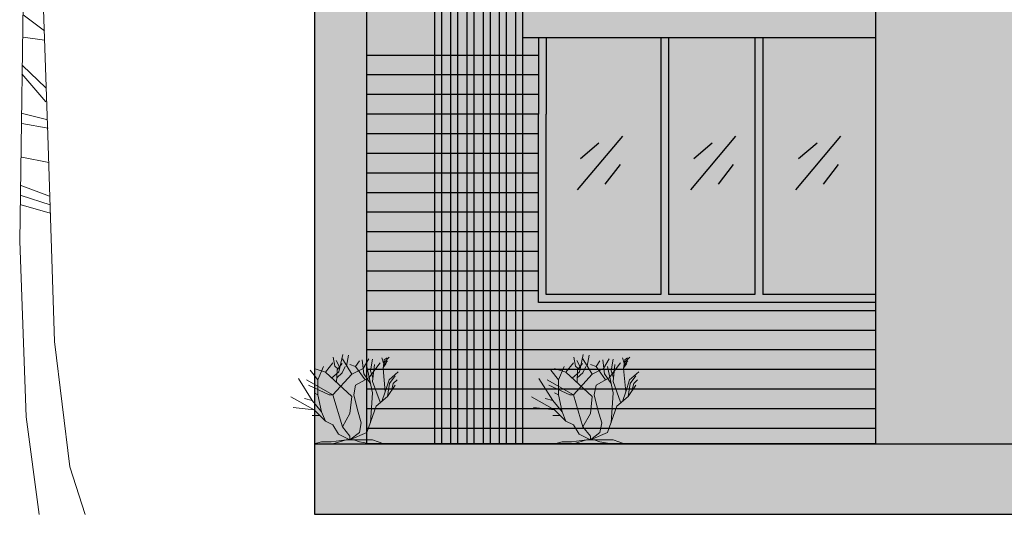
# Model space of a CAD drawing. Units: inches. Extents: x 13 to 1693, y -7 to 1519.
# Tile 5 of 10: x 41 to 292, y 1195 to 1321. Entities that reach past the tile are written whole.
import ezdxf

# ---------------------------------------------------------------- set-up
doc = ezdxf.new("R2010")
doc.units = ezdxf.units.IN
doc.header["$MEASUREMENT"] = 0
for name, color, linetype, lineweight in [('A-ELEV', 7, 'Continuous', 25), ('A-ELEV-PATT', 8, 'Continuous', 13), ('TREE', 102, 'Continuous', 18)]:
    doc.layers.add(name, color=color, linetype=linetype, lineweight=lineweight)

# ---------------------------------------------------------------- blocks, each defined once
blk = doc.blocks.new('*U29')
for p, q in [((-4.081, 127.298), (1.31, 123.246)), ((-4.081, 121.578), (1.31, 120.863)), ((-4.267, 114.428), (1.682, 108.708)), ((-4.453, 112.283), (1.682, 105.133)), ((-4.639, 102.273), (1.868, 100.604)), ((-4.453, 99.651), (2.24, 98.459)), ((-4.453, 91.071), (2.426, 89.641)), ((-4.825, 83.921), (2.612, 81.061)), ((-4.639, 81.299), (2.797, 78.916)), ((-4.639, 78.916), (2.797, 76.771))]:
    blk.add_line(p, q)
for points in [[(-2.363, 170.553), (-3.88, 148.505), (-4.988, 69.634), (-3.325, 24.869), (0, 0)], [(-0.116, 162.848), (0.554, 143.532), (2.217, 96.635), (3.88, 44.054), (7.76, 12.079), (11.64, 0)]]:
    blk.add_lwpolyline(points)
blk = doc.blocks.new('*U30')
for p, q in [((-11.433, 18.289), (-10.457, 22.749)), ((-9.48, 19.775), (-8.992, 22.592)), ((-14.88, 18.24), (-12.96, 20.64)), ((-12.471, 19.775), (-12.898, 22.044)), ((-11.28, 19.619), (-12.104, 21.184)), ((-11.921, 18.836), (-10.64, 20.401)), ((-8.16, 17.76), (-10.56, 21.6)), ((-7.2, 19.68), (-8.64, 20.16)), ((-7.2, 19.68), (-6.24, 21.12)), ((-5.086, 17.741), (-5.513, 21.34)), ((-5.28, 19.2), (-3.84, 21.6)), ((-3.84, 16.8), (-0.96, 20.64)), ((-3.377, 18.602), (-2.888, 21.575)), ((-2.88, 15.84), (-2.4, 20.16)), ((-0.508, 21.888), (-0.081, 20.558)), ((-0.203, 19.149), (0.102, 21.34)), ((-0.142, 19.384), (0.59, 20.401)), ((-0.02, 20.01), (0.896, 21.105)), ((0.041, 20.714), (1.384, 22.044)), ((0.102, 21.34), (0.835, 21.888)), ((-16.8, 16.32), (-18.72, 18.72)), ((-14.88, 18.24), (-17.76, 19.2)), ((-16.8, 16.32), (-15.36, 19.68)), ((-8.16, 12), (-14.88, 18.24)), ((-13.325, 16.724), (-11.433, 18.289)), ((-12.96, 12.48), (-8.16, 17.76)), ((-11.677, 19.071), (-12.471, 19.775)), ((-12.043, 15.628), (-11.921, 18.836)), ((-11.982, 16.802), (-10.579, 18.054)), ((-10.579, 18.054), (-9.846, 19.697)), ((-8.16, 17.76), (-5.28, 19.2)), ((-4.8, 16.32), (-7.2, 19.68)), ((-3.377, 15.315), (-5.086, 17.819)), ((-2.88, 12.96), (-4.32, 19.68)), ((-2.766, 16.802), (-3.377, 18.602)), ((0.346, 13.203), (-0.203, 19.149)), ((1.323, 16.254), (3.642, 18.289)), ((-18.24, 11.04), (-21.755, 16.655)), ((-12.96, 12.48), (-19.68, 16.32)), ((-16.8, 12.48), (-16.8, 16.32)), ((-7.2, 14.88), (-3.84, 16.8)), ((-0.96, 10.56), (-2.88, 15.84)), ((0.346, 13.203), (1.323, 16.254)), ((0.96, 12), (1.44, 15.36)), ((1.44, 15.36), (2.88, 17.28)), ((1.92, 13.44), (2.4, 15.36)), ((2.4, 15.36), (3.36, 16.32)), ((-13.92, 12.48), (-19.2, 14.88)), ((-16.8, 12.48), (-17.76, 12.96)), ((-7.68, 12.48), (-7.2, 14.88)), ((-3.36, 5.28), (-2.88, 12.96)), ((-0.48, 10.8), (0.346, 13.203)), ((0.96, 12), (2.88, 14.88)), ((-17.76, 8.64), (-23.663, 11.961)), ((-18.24, 11.04), (-20.16, 11.52)), ((-15.84, 8.16), (-18.24, 11.04)), ((-15.84, 8.16), (-16.8, 12.48)), ((-12.96, 12.48), (-13.92, 12.48)), ((-10.56, 4.32), (-12.96, 12.48)), ((-8.64, 7.68), (-8.16, 12)), ((-6.72, 8.64), (-7.68, 12.48)), ((-1.92, 9.6), (0.96, 12)), ((-17.76, 8.64), (-23.128, 9.222)), ((-14.88, 5.76), (-17.76, 8.64)), ((-14.88, 5.76), (-15.84, 8.16)), ((-10.56, 4.32), (-8.64, 7.68)), ((-5.76, 5.28), (-6.72, 8.64)), ((-4.32, 2.88), (-1.92, 9.6)), ((-16.32, 7.2), (-18.24, 7.2)), ((-12.96, 4.8), (-14.88, 5.76)), ((-6.24, 2.88), (-5.76, 5.28)), ((-11.52, 2.4), (-12.96, 4.8)), ((-8.64, 1.92), (-10.56, 4.32)), ((-8.64, 0.96), (-4.32, 2.88)), ((-8.64, 0.96), (-6.24, 2.88)), ((-15.84, 0.48), (-17.76, 0)), ((-13.44, 0.48), (-15.84, 0.48)), ((-9.6, 0.96), (-13.44, 0.48)), ((-9.6, 0.96), (-12.96, 0)), ((-8.64, 0.96), (-11.52, 2.4)), ((-9.6, 0.96), (-7.68, 0.96)), ((-8.64, 0.96), (-8.64, 1.92)), ((-8.64, 0.96), (-2.88, 0.96)), ((-7.68, 0.96), (-6.24, 0.48)), ((-6.24, 0.48), (-3.36, 0)), ((-2.88, 0.96), (0, 0))]:
    blk.add_line(p, q)

msp = doc.modelspace()

# ---------------------------------------------------------------- hatches: boundary and pattern name
at = {"layer": 'A-ELEV-PATT', "transparency": 33554664}
h = msp.add_hatch(color=256, dxfattribs=at)
h.dxf.hatch_style = 1
h.paths.add_polyline_path([(161.14, 1507.23), (159.26, 1507.23), (159.26, 1457.61), (161.14, 1457.61)])
h.paths.add_polyline_path([(161.14, 1510.4), (159.26, 1512.79), (159.26, 1507.23), (161.14, 1507.23)])
h.paths.add_polyline_path([(165.27, 1510.4), (163.39, 1512.79), (163.39, 1507.23), (165.27, 1507.23)])
h.paths.add_polyline_path([(169.4, 1510.4), (167.53, 1512.79), (167.53, 1507.23), (169.4, 1507.23)])
h.paths.add_polyline_path([(157.01, 1510.4), (155.13, 1512.79), (155.13, 1507.23), (157.01, 1507.23)])
h.paths.add_polyline_path([(152.87, 1510.4), (151, 1512.79), (151, 1507.23), (152.87, 1507.23)])
h.paths.add_polyline_path([(148.74, 1510.4), (146.87, 1512.79), (146.87, 1507.23), (148.74, 1507.23)])
h.paths.add_polyline_path([(148.74, 1507.23), (146.87, 1507.23), (146.87, 1457.61), (148.74, 1457.61)])
h.paths.add_polyline_path([(152.87, 1507.23), (151, 1507.23), (151, 1457.61), (152.87, 1457.61)])
h.paths.add_polyline_path([(157.01, 1507.23), (155.13, 1507.23), (155.13, 1457.61), (157.01, 1457.61)])
h.paths.add_polyline_path([(165.27, 1507.23), (163.39, 1507.23), (163.39, 1457.61), (165.27, 1457.61)])
h.paths.add_polyline_path([(169.4, 1507.23), (167.53, 1507.23), (167.53, 1457.61), (169.4, 1457.61)])
h.paths.add_polyline_path([(157.01, 1457.61), (155.13, 1457.61), (155.13, 1213.23), (157.01, 1213.23)])
h.paths.add_polyline_path([(161.14, 1457.61), (159.26, 1457.61), (159.26, 1213.23), (161.14, 1213.23)])
h.paths.add_polyline_path([(165.27, 1457.61), (163.39, 1457.61), (163.39, 1213.23), (165.27, 1213.23)])
h.paths.add_polyline_path([(169.4, 1457.61), (167.53, 1457.61), (167.53, 1213.23), (169.4, 1213.23)])
h.paths.add_polyline_path([(152.87, 1457.61), (151, 1457.61), (151, 1213.23), (152.87, 1213.23)])
h.paths.add_polyline_path([(148.74, 1457.61), (146.87, 1457.61), (146.87, 1213.23), (148.74, 1213.23)])
at = {"layer": 'A-ELEV-PATT'}
h = msp.add_hatch(color=256, dxfattribs=at)
h.dxf.hatch_style = 1
h.paths.add_polyline_path([(534.67, 1493.81), (311.73, 1493.81), (311.73, 1507.23), (169.4, 1507.23), (169.4, 1457.61), (259.19, 1457.61), (259.19, 1213.23), (294.63, 1213.23), (294.63, 1485.7), (299.21, 1485.7), (534.67, 1485.7)])
h.paths.add_polyline_path([(534.67, 1481.12), (299.21, 1481.12), (299.21, 1213.23), (314.45, 1213.23), (314.45, 1459.23), (520.13, 1459.23)], flags=17)
h.paths.add_polyline_path([(146.87, 1507.23), (116.45, 1507.23), (116.45, 1339.23), (116.45, 1213.23), (129.66, 1213.23), (129.66, 1457.61), (146.87, 1457.61)])
h.paths.add_polyline_path([(151, 1507.23), (148.74, 1507.23), (148.74, 1457.61), (151, 1457.61)])
h.paths.add_polyline_path([(155.13, 1507.23), (152.87, 1507.23), (152.87, 1457.61), (155.13, 1457.61)])
h.paths.add_polyline_path([(159.26, 1507.23), (157.01, 1507.23), (157.01, 1457.61), (159.26, 1457.61)])
h.paths.add_polyline_path([(163.39, 1507.23), (161.14, 1507.23), (161.14, 1457.61), (163.39, 1457.61)])
h.paths.add_polyline_path([(167.53, 1507.23), (165.27, 1507.23), (165.27, 1457.61), (167.53, 1457.61)])
h = msp.add_hatch(color=256, dxfattribs=at)
h.dxf.hatch_style = 1
h.paths.add_polyline_path([(259.19, 1457.61), (169.4, 1457.61), (169.4, 1453.8), (259.19, 1453.8)])
h.paths.add_polyline_path([(259.19, 1448.8), (169.4, 1448.8), (169.4, 1443.8), (259.19, 1443.8)])
h.paths.add_polyline_path([(259.19, 1438.8), (169.4, 1438.8), (169.4, 1433.8), (259.19, 1433.8)])
h.paths.add_polyline_path([(259.19, 1428.8), (169.4, 1428.8), (169.4, 1423.8), (259.19, 1423.8)])
h.paths.add_polyline_path([(146.87, 1457.61), (129.66, 1457.61), (129.66, 1453.8), (146.87, 1453.8)])
h.paths.add_polyline_path([(146.87, 1448.8), (129.66, 1448.8), (129.66, 1443.8), (146.87, 1443.8)])
h.paths.add_polyline_path([(146.87, 1438.8), (129.66, 1438.8), (129.66, 1433.8), (146.87, 1433.8)])
h.paths.add_polyline_path([(146.87, 1428.8), (129.66, 1428.8), (129.66, 1423.8), (146.87, 1423.8)])
h.paths.add_polyline_path([(151, 1457.61), (148.74, 1457.61), (148.74, 1453.8), (151, 1453.8)])
h.paths.add_polyline_path([(155.13, 1457.61), (152.87, 1457.61), (152.87, 1453.8), (155.13, 1453.8)])
h.paths.add_polyline_path([(159.26, 1457.61), (157.01, 1457.61), (157.01, 1453.8), (159.26, 1453.8)])
h.paths.add_polyline_path([(163.39, 1457.61), (161.14, 1457.61), (161.14, 1453.8), (163.39, 1453.8)])
h.paths.add_polyline_path([(167.53, 1457.61), (165.27, 1457.61), (165.27, 1453.8), (167.53, 1453.8)])
h.paths.add_polyline_path([(167.53, 1448.8), (165.27, 1448.8), (165.27, 1443.8), (167.53, 1443.8)])
h.paths.add_polyline_path([(163.39, 1448.8), (161.14, 1448.8), (161.14, 1443.8), (163.39, 1443.8)])
h.paths.add_polyline_path([(159.26, 1448.8), (157.01, 1448.8), (157.01, 1443.8), (159.26, 1443.8)])
h.paths.add_polyline_path([(155.13, 1448.8), (152.87, 1448.8), (152.87, 1443.8), (155.13, 1443.8)])
h.paths.add_polyline_path([(151, 1448.8), (148.74, 1448.8), (148.74, 1443.8), (151, 1443.8)])
h.paths.add_polyline_path([(151, 1438.8), (148.74, 1438.8), (148.74, 1433.8), (151, 1433.8)])
h.paths.add_polyline_path([(155.13, 1438.8), (152.87, 1438.8), (152.87, 1433.8), (155.13, 1433.8)])
h.paths.add_polyline_path([(159.26, 1438.8), (157.01, 1438.8), (157.01, 1433.8), (159.26, 1433.8)])
h.paths.add_polyline_path([(163.39, 1438.8), (161.14, 1438.8), (161.14, 1433.8), (163.39, 1433.8)])
h.paths.add_polyline_path([(167.53, 1438.8), (165.27, 1438.8), (165.27, 1433.8), (167.53, 1433.8)])
h.paths.add_polyline_path([(167.53, 1428.8), (165.27, 1428.8), (165.27, 1423.8), (167.53, 1423.8)])
h.paths.add_polyline_path([(163.39, 1428.8), (161.14, 1428.8), (161.14, 1423.8), (163.39, 1423.8)])
h.paths.add_polyline_path([(159.26, 1428.8), (157.01, 1428.8), (157.01, 1423.8), (159.26, 1423.8)])
h.paths.add_polyline_path([(155.13, 1428.8), (152.87, 1428.8), (152.87, 1423.8), (155.13, 1423.8)])
h.paths.add_polyline_path([(151, 1428.8), (148.74, 1428.8), (148.74, 1423.8), (151, 1423.8)])
h.paths.add_polyline_path([(146.87, 1418.8), (129.66, 1418.8), (129.66, 1413.8), (146.87, 1413.8)])
h.paths.add_polyline_path([(146.87, 1408.8), (129.66, 1408.8), (129.66, 1403.8), (146.87, 1403.8)])
h.paths.add_polyline_path([(146.87, 1398.8), (129.66, 1398.8), (129.66, 1393.8), (146.87, 1393.8)])
h.paths.add_polyline_path([(146.87, 1388.8), (129.66, 1388.8), (129.66, 1383.8), (146.87, 1383.8)])
h.paths.add_polyline_path([(146.87, 1378.8), (129.66, 1378.8), (129.66, 1373.8), (146.87, 1373.8)])
h.paths.add_polyline_path([(146.87, 1368.8), (129.66, 1368.8), (129.66, 1363.8), (146.87, 1363.8)])
h.paths.add_polyline_path([(146.87, 1358.8), (129.66, 1358.8), (129.66, 1353.8), (146.87, 1353.8)])
h.paths.add_polyline_path([(146.87, 1348.8), (129.66, 1348.8), (129.66, 1343.8), (146.87, 1343.8)])
h.paths.add_polyline_path([(146.87, 1338.8), (129.66, 1338.8), (129.66, 1333.8), (146.87, 1333.8)])
h.paths.add_polyline_path([(146.87, 1328.8), (129.66, 1328.8), (129.66, 1323.8), (146.87, 1323.8)])
h.paths.add_polyline_path([(146.87, 1318.8), (129.66, 1318.8), (129.66, 1312.21), (146.87, 1312.21)])
h.paths.add_polyline_path([(146.87, 1307.21), (129.66, 1307.21), (129.66, 1302.21), (146.87, 1302.21)])
h.paths.add_polyline_path([(146.87, 1297.21), (129.66, 1297.21), (129.66, 1292.21), (146.87, 1292.21)])
h.paths.add_polyline_path([(146.87, 1287.21), (129.66, 1287.21), (129.66, 1282.21), (146.87, 1282.21)])
h.paths.add_polyline_path([(146.87, 1277.21), (129.66, 1277.21), (129.66, 1272.21), (146.87, 1272.21)])
h.paths.add_polyline_path([(146.87, 1267.21), (129.66, 1267.21), (129.66, 1262.21), (146.87, 1262.21)])
h.paths.add_polyline_path([(146.87, 1257.21), (129.66, 1257.21), (129.66, 1252.21), (146.87, 1252.21)])
h.paths.add_polyline_path([(146.87, 1247.21), (129.66, 1247.21), (129.66, 1242.21), (146.87, 1242.21)])
h = msp.add_hatch(color=256, dxfattribs=at)
h.dxf.hatch_style = 1
h.paths.add_polyline_path([(259.19, 1453.8), (169.4, 1453.8), (169.4, 1448.8), (259.19, 1448.8)])
h.paths.add_polyline_path([(259.19, 1443.8), (169.4, 1443.8), (169.4, 1438.8), (259.19, 1438.8)])
h.paths.add_polyline_path([(259.19, 1433.8), (169.4, 1433.8), (169.4, 1428.8), (259.19, 1428.8)])
h.paths.add_polyline_path([(146.87, 1453.8), (129.66, 1453.8), (129.66, 1448.8), (146.87, 1448.8)])
h.paths.add_polyline_path([(146.87, 1443.8), (129.66, 1443.8), (129.66, 1438.8), (146.87, 1438.8)])
h.paths.add_polyline_path([(146.87, 1433.8), (129.66, 1433.8), (129.66, 1428.8), (146.87, 1428.8)])
h.paths.add_polyline_path([(146.87, 1423.8), (129.66, 1423.8), (129.66, 1418.8), (146.87, 1418.8)])
h.paths.add_polyline_path([(146.87, 1413.8), (129.66, 1413.8), (129.66, 1408.8), (146.87, 1408.8)])
h.paths.add_polyline_path([(146.87, 1403.8), (129.66, 1403.8), (129.66, 1398.8), (146.87, 1398.8)])
h.paths.add_polyline_path([(146.87, 1393.8), (129.66, 1393.8), (129.66, 1388.8), (146.87, 1388.8)])
h.paths.add_polyline_path([(146.87, 1383.8), (129.66, 1383.8), (129.66, 1378.8), (146.87, 1378.8)])
h.paths.add_polyline_path([(146.87, 1373.8), (129.66, 1373.8), (129.66, 1368.8), (146.87, 1368.8)])
h.paths.add_polyline_path([(146.87, 1363.8), (129.66, 1363.8), (129.66, 1358.8), (146.87, 1358.8)])
h.paths.add_polyline_path([(146.87, 1353.8), (129.66, 1353.8), (129.66, 1348.8), (146.87, 1348.8)])
h.paths.add_polyline_path([(146.87, 1343.8), (129.66, 1343.8), (129.66, 1338.8), (146.87, 1338.8)])
h.paths.add_polyline_path([(146.87, 1333.8), (129.66, 1333.8), (129.66, 1328.8), (146.87, 1328.8)])
h.paths.add_polyline_path([(146.87, 1323.8), (129.66, 1323.8), (129.66, 1318.8), (146.87, 1318.8)])
h.paths.add_polyline_path([(146.87, 1312.21), (129.66, 1312.21), (129.66, 1307.21), (146.87, 1307.21)])
h.paths.add_polyline_path([(146.87, 1302.21), (129.66, 1302.21), (129.66, 1297.21), (146.87, 1297.21)])
h.paths.add_polyline_path([(146.87, 1292.21), (129.66, 1292.21), (129.66, 1287.21), (146.87, 1287.21)])
h.paths.add_polyline_path([(146.87, 1282.21), (129.66, 1282.21), (129.66, 1277.21), (146.87, 1277.21)])
h.paths.add_polyline_path([(146.87, 1272.21), (129.66, 1272.21), (129.66, 1267.21), (146.87, 1267.21)])
h.paths.add_polyline_path([(146.87, 1262.21), (129.66, 1262.21), (129.66, 1257.21), (146.87, 1257.21)])
h.paths.add_polyline_path([(146.87, 1252.21), (129.66, 1252.21), (129.66, 1247.21), (146.87, 1247.21)])
h.paths.add_polyline_path([(146.87, 1242.21), (129.66, 1242.21), (129.66, 1237.21), (146.87, 1237.21)])
h.paths.add_polyline_path([(146.87, 1232.21), (129.66, 1232.21), (129.66, 1227.21), (146.87, 1227.21)])
h.paths.add_polyline_path([(146.87, 1222.21), (129.66, 1222.21), (129.66, 1217.21), (146.87, 1217.21)])
h.paths.add_polyline_path([(259.19, 1242.21), (169.4, 1242.21), (169.4, 1237.21), (259.19, 1237.21)])
h.paths.add_polyline_path([(259.19, 1232.21), (169.4, 1232.21), (169.4, 1227.21), (259.19, 1227.21)])
h.paths.add_polyline_path([(259.19, 1222.21), (169.4, 1222.21), (169.4, 1217.21), (259.19, 1217.21)])
h = msp.add_hatch(color=256, dxfattribs=at)
h.dxf.hatch_style = 1
h.paths.add_polyline_path([(173.34, 1282.21), (169.4, 1282.21), (169.4, 1277.21), (173.34, 1277.21)])
h.paths.add_polyline_path([(173.34, 1292.21), (169.4, 1292.21), (169.4, 1287.21), (173.34, 1287.21)])
h.paths.add_polyline_path([(173.34, 1272.21), (169.4, 1272.21), (169.4, 1267.21), (173.34, 1267.21)])
h.paths.add_polyline_path([(173.34, 1262.21), (169.4, 1262.21), (169.4, 1257.21), (173.34, 1257.21)])
h.paths.add_polyline_path([(173.34, 1312.21), (169.4, 1312.21), (169.4, 1307.21), (173.34, 1307.21)])
h.paths.add_polyline_path([(173.34, 1302.21), (169.4, 1302.21), (169.4, 1297.21), (173.34, 1297.21)])
h.paths.add_polyline_path([(167.53, 1323.8), (165.27, 1323.8), (165.27, 1318.8), (167.53, 1318.8)])
h.paths.add_polyline_path([(167.53, 1333.8), (165.27, 1333.8), (165.27, 1328.8), (167.53, 1328.8)])
h.paths.add_polyline_path([(163.39, 1333.8), (161.14, 1333.8), (161.14, 1328.8), (163.39, 1328.8)])
h.paths.add_polyline_path([(159.26, 1333.8), (157.01, 1333.8), (157.01, 1328.8), (159.26, 1328.8)])
h.paths.add_polyline_path([(155.13, 1333.8), (152.87, 1333.8), (152.87, 1328.8), (155.13, 1328.8)])
h.paths.add_polyline_path([(151, 1333.8), (148.74, 1333.8), (148.74, 1328.8), (151, 1328.8)])
h.paths.add_polyline_path([(151, 1323.8), (148.74, 1323.8), (148.74, 1318.8), (151, 1318.8)])
h.paths.add_polyline_path([(155.13, 1323.8), (152.87, 1323.8), (152.87, 1318.8), (155.13, 1318.8)])
h.paths.add_polyline_path([(159.26, 1323.8), (157.01, 1323.8), (157.01, 1318.8), (159.26, 1318.8)])
h.paths.add_polyline_path([(163.39, 1323.8), (161.14, 1323.8), (161.14, 1318.8), (163.39, 1318.8)])
h.paths.add_polyline_path([(163.39, 1312.21), (161.14, 1312.21), (161.14, 1307.21), (163.39, 1307.21)])
h.paths.add_polyline_path([(167.53, 1312.21), (165.27, 1312.21), (165.27, 1307.21), (167.53, 1307.21)])
h.paths.add_polyline_path([(167.53, 1302.21), (165.27, 1302.21), (165.27, 1297.21), (167.53, 1297.21)])
h.paths.add_polyline_path([(167.53, 1292.21), (165.27, 1292.21), (165.27, 1287.21), (167.53, 1287.21)])
h.paths.add_polyline_path([(163.39, 1292.21), (161.14, 1292.21), (161.14, 1287.21), (163.39, 1287.21)])
h.paths.add_polyline_path([(163.39, 1302.21), (161.14, 1302.21), (161.14, 1297.21), (163.39, 1297.21)])
h.paths.add_polyline_path([(159.26, 1302.21), (157.01, 1302.21), (157.01, 1297.21), (159.26, 1297.21)])
h.paths.add_polyline_path([(159.26, 1312.21), (157.01, 1312.21), (157.01, 1307.21), (159.26, 1307.21)])
h.paths.add_polyline_path([(155.13, 1312.21), (152.87, 1312.21), (152.87, 1307.21), (155.13, 1307.21)])
h.paths.add_polyline_path([(151, 1312.21), (148.74, 1312.21), (148.74, 1307.21), (151, 1307.21)])
h.paths.add_polyline_path([(151, 1302.21), (148.74, 1302.21), (148.74, 1297.21), (151, 1297.21)])
h.paths.add_polyline_path([(155.13, 1302.21), (152.87, 1302.21), (152.87, 1297.21), (155.13, 1297.21)])
h.paths.add_polyline_path([(155.13, 1292.21), (152.87, 1292.21), (152.87, 1287.21), (155.13, 1287.21)])
h.paths.add_polyline_path([(151, 1292.21), (148.74, 1292.21), (148.74, 1287.21), (151, 1287.21)])
h.paths.add_polyline_path([(159.26, 1292.21), (157.01, 1292.21), (157.01, 1287.21), (159.26, 1287.21)])
h.paths.add_polyline_path([(159.26, 1282.21), (157.01, 1282.21), (157.01, 1277.21), (159.26, 1277.21)])
h.paths.add_polyline_path([(163.39, 1282.21), (161.14, 1282.21), (161.14, 1277.21), (163.39, 1277.21)])
h.paths.add_polyline_path([(167.53, 1282.21), (165.27, 1282.21), (165.27, 1277.21), (167.53, 1277.21)])
h.paths.add_polyline_path([(155.13, 1282.21), (152.87, 1282.21), (152.87, 1277.21), (155.13, 1277.21)])
h.paths.add_polyline_path([(151, 1282.21), (148.74, 1282.21), (148.74, 1277.21), (151, 1277.21)])
h.paths.add_polyline_path([(151, 1272.21), (148.74, 1272.21), (148.74, 1267.21), (151, 1267.21)])
h.paths.add_polyline_path([(155.13, 1272.21), (152.87, 1272.21), (152.87, 1267.21), (155.13, 1267.21)])
h.paths.add_polyline_path([(159.26, 1272.21), (157.01, 1272.21), (157.01, 1267.21), (159.26, 1267.21)])
h.paths.add_polyline_path([(163.39, 1272.21), (161.14, 1272.21), (161.14, 1267.21), (163.39, 1267.21)])
h.paths.add_polyline_path([(167.53, 1272.21), (165.27, 1272.21), (165.27, 1267.21), (167.53, 1267.21)])
h.paths.add_polyline_path([(167.53, 1262.21), (165.27, 1262.21), (165.27, 1257.21), (167.53, 1257.21)])
h.paths.add_polyline_path([(163.39, 1262.21), (161.14, 1262.21), (161.14, 1257.21), (163.39, 1257.21)])
h.paths.add_polyline_path([(163.39, 1252.21), (161.14, 1252.21), (161.14, 1247.21), (163.39, 1247.21)])
h.paths.add_polyline_path([(159.26, 1252.21), (157.01, 1252.21), (157.01, 1247.21), (159.26, 1247.21)])
h.paths.add_polyline_path([(159.26, 1262.21), (157.01, 1262.21), (157.01, 1257.21), (159.26, 1257.21)])
h.paths.add_polyline_path([(155.13, 1262.21), (152.87, 1262.21), (152.87, 1257.21), (155.13, 1257.21)])
h.paths.add_polyline_path([(151, 1262.21), (148.74, 1262.21), (148.74, 1257.21), (151, 1257.21)])
h.paths.add_polyline_path([(151, 1252.21), (148.74, 1252.21), (148.74, 1247.21), (151, 1247.21)])
h.paths.add_polyline_path([(155.13, 1252.21), (152.87, 1252.21), (152.87, 1247.21), (155.13, 1247.21)])
h.paths.add_polyline_path([(151, 1242.21), (148.74, 1242.21), (148.74, 1237.21), (151, 1237.21)])
h.paths.add_polyline_path([(155.13, 1242.21), (152.87, 1242.21), (152.87, 1237.21), (155.13, 1237.21)])
h.paths.add_polyline_path([(159.26, 1242.21), (157.01, 1242.21), (157.01, 1237.21), (159.26, 1237.21)])
h.paths.add_polyline_path([(163.39, 1242.21), (161.14, 1242.21), (161.14, 1237.21), (163.39, 1237.21)])
h.paths.add_polyline_path([(173.34, 1363.8), (169.4, 1363.8), (169.4, 1358.8), (173.34, 1358.8)])
h.paths.add_polyline_path([(173.34, 1373.8), (169.4, 1373.8), (169.4, 1368.8), (173.34, 1368.8)])
h.paths.add_polyline_path([(173.34, 1381.23), (173.34, 1383.8), (169.4, 1383.8), (169.4, 1378.8), (173.34, 1378.8)])
h.paths.add_polyline_path([(173.34, 1393.8), (169.4, 1393.8), (169.4, 1388.8), (173.34, 1388.8)])
h.paths.add_polyline_path([(173.34, 1403.8), (169.4, 1403.8), (169.4, 1398.8), (173.34, 1398.8)])
h.paths.add_polyline_path([(173.34, 1413.8), (169.4, 1413.8), (169.4, 1408.8), (173.34, 1408.8)])
h.paths.add_polyline_path([(167.53, 1383.8), (165.27, 1383.8), (165.27, 1378.8), (167.53, 1378.8)])
h.paths.add_polyline_path([(167.53, 1373.8), (165.27, 1373.8), (165.27, 1368.8), (167.53, 1368.8)])
h.paths.add_polyline_path([(167.53, 1363.8), (165.27, 1363.8), (165.27, 1358.8), (167.53, 1358.8)])
h.paths.add_polyline_path([(167.53, 1353.8), (165.27, 1353.8), (165.27, 1348.8), (167.53, 1348.8)])
h.paths.add_polyline_path([(163.39, 1353.8), (161.14, 1353.8), (161.14, 1348.8), (163.39, 1348.8)])
h.paths.add_polyline_path([(163.39, 1363.8), (161.14, 1363.8), (161.14, 1358.8), (163.39, 1358.8)])
h.paths.add_polyline_path([(163.39, 1373.8), (161.14, 1373.8), (161.14, 1368.8), (163.39, 1368.8)])
h.paths.add_polyline_path([(163.39, 1383.8), (161.14, 1383.8), (161.14, 1378.8), (163.39, 1378.8)])
h.paths.add_polyline_path([(163.39, 1393.8), (161.14, 1393.8), (161.14, 1388.8), (163.39, 1388.8)])
h.paths.add_polyline_path([(163.39, 1403.8), (161.14, 1403.8), (161.14, 1398.8), (163.39, 1398.8)])
h.paths.add_polyline_path([(167.53, 1403.8), (165.27, 1403.8), (165.27, 1398.8), (167.53, 1398.8)])
h.paths.add_polyline_path([(167.53, 1393.8), (165.27, 1393.8), (165.27, 1388.8), (167.53, 1388.8)])
h.paths.add_polyline_path([(167.53, 1413.8), (165.27, 1413.8), (165.27, 1408.8), (167.53, 1408.8)])
h.paths.add_polyline_path([(163.39, 1413.8), (161.14, 1413.8), (161.14, 1408.8), (163.39, 1408.8)])
h.paths.add_polyline_path([(159.26, 1413.8), (157.01, 1413.8), (157.01, 1408.8), (159.26, 1408.8)])
h.paths.add_polyline_path([(155.13, 1413.8), (152.87, 1413.8), (152.87, 1408.8), (155.13, 1408.8)])
h.paths.add_polyline_path([(151, 1413.8), (148.74, 1413.8), (148.74, 1408.8), (151, 1408.8)])
h.paths.add_polyline_path([(151, 1403.8), (148.74, 1403.8), (148.74, 1398.8), (151, 1398.8)])
h.paths.add_polyline_path([(155.13, 1403.8), (152.87, 1403.8), (152.87, 1398.8), (155.13, 1398.8)])
h.paths.add_polyline_path([(159.26, 1403.8), (157.01, 1403.8), (157.01, 1398.8), (159.26, 1398.8)])
h.paths.add_polyline_path([(159.26, 1393.8), (157.01, 1393.8), (157.01, 1388.8), (159.26, 1388.8)])
h.paths.add_polyline_path([(155.13, 1393.8), (152.87, 1393.8), (152.87, 1388.8), (155.13, 1388.8)])
h.paths.add_polyline_path([(151, 1393.8), (148.74, 1393.8), (148.74, 1388.8), (151, 1388.8)])
h.paths.add_polyline_path([(151, 1383.8), (148.74, 1383.8), (148.74, 1378.8), (151, 1378.8)])
h.paths.add_polyline_path([(155.13, 1383.8), (152.87, 1383.8), (152.87, 1378.8), (155.13, 1378.8)])
h.paths.add_polyline_path([(159.26, 1383.8), (157.01, 1383.8), (157.01, 1378.8), (159.26, 1378.8)])
h.paths.add_polyline_path([(159.26, 1373.8), (157.01, 1373.8), (157.01, 1368.8), (159.26, 1368.8)])
h.paths.add_polyline_path([(155.13, 1373.8), (152.87, 1373.8), (152.87, 1368.8), (155.13, 1368.8)])
h.paths.add_polyline_path([(151, 1373.8), (148.74, 1373.8), (148.74, 1368.8), (151, 1368.8)])
h.paths.add_polyline_path([(151, 1363.8), (148.74, 1363.8), (148.74, 1358.8), (151, 1358.8)])
h.paths.add_polyline_path([(155.13, 1363.8), (152.87, 1363.8), (152.87, 1358.8), (155.13, 1358.8)])
h.paths.add_polyline_path([(159.26, 1363.8), (157.01, 1363.8), (157.01, 1358.8), (159.26, 1358.8)])
h.paths.add_polyline_path([(159.26, 1353.8), (157.01, 1353.8), (157.01, 1348.8), (159.26, 1348.8)])
h.paths.add_polyline_path([(155.13, 1353.8), (152.87, 1353.8), (152.87, 1348.8), (155.13, 1348.8)])
h.paths.add_polyline_path([(151, 1353.8), (148.74, 1353.8), (148.74, 1348.8), (151, 1348.8)])
h.paths.add_polyline_path([(151, 1343.8), (148.74, 1343.8), (148.74, 1338.8), (151, 1338.8)])
h.paths.add_polyline_path([(155.13, 1343.8), (152.87, 1343.8), (152.87, 1338.8), (155.13, 1338.8)])
h.paths.add_polyline_path([(159.26, 1343.8), (157.01, 1343.8), (157.01, 1338.8), (159.26, 1338.8)])
h.paths.add_polyline_path([(163.39, 1343.8), (161.14, 1343.8), (161.14, 1338.8), (163.39, 1338.8)])
h.paths.add_polyline_path([(167.53, 1343.8), (165.27, 1343.8), (165.27, 1338.8), (167.53, 1338.8)])
h.paths.add_polyline_path([(151, 1453.8), (148.74, 1453.8), (148.74, 1448.8), (151, 1448.8)])
h.paths.add_polyline_path([(155.13, 1453.8), (152.87, 1453.8), (152.87, 1448.8), (155.13, 1448.8)])
h.paths.add_polyline_path([(159.26, 1453.8), (157.01, 1453.8), (157.01, 1448.8), (159.26, 1448.8)])
h.paths.add_polyline_path([(163.39, 1453.8), (161.14, 1453.8), (161.14, 1448.8), (163.39, 1448.8)])
h.paths.add_polyline_path([(167.53, 1453.8), (165.27, 1453.8), (165.27, 1448.8), (167.53, 1448.8)])
h.paths.add_polyline_path([(167.53, 1443.8), (165.27, 1443.8), (165.27, 1438.8), (167.53, 1438.8)])
h.paths.add_polyline_path([(163.39, 1443.8), (161.14, 1443.8), (161.14, 1438.8), (163.39, 1438.8)])
h.paths.add_polyline_path([(159.26, 1443.8), (157.01, 1443.8), (157.01, 1438.8), (159.26, 1438.8)])
h.paths.add_polyline_path([(155.13, 1443.8), (152.87, 1443.8), (152.87, 1438.8), (155.13, 1438.8)])
h.paths.add_polyline_path([(151, 1443.8), (148.74, 1443.8), (148.74, 1438.8), (151, 1438.8)])
h.paths.add_polyline_path([(151, 1433.8), (148.74, 1433.8), (148.74, 1428.8), (151, 1428.8)])
h.paths.add_polyline_path([(155.13, 1433.8), (152.87, 1433.8), (152.87, 1428.8), (155.13, 1428.8)])
h.paths.add_polyline_path([(159.26, 1433.8), (157.01, 1433.8), (157.01, 1428.8), (159.26, 1428.8)])
h.paths.add_polyline_path([(163.39, 1433.8), (161.14, 1433.8), (161.14, 1428.8), (163.39, 1428.8)])
h.paths.add_polyline_path([(167.53, 1433.8), (165.27, 1433.8), (165.27, 1428.8), (167.53, 1428.8)])
h.paths.add_polyline_path([(173.34, 1423.23), (249.37, 1423.23), (259.19, 1423.23), (259.19, 1423.8), (169.4, 1423.8), (169.4, 1418.8), (173.34, 1418.8)])
h.paths.add_polyline_path([(167.53, 1423.8), (165.27, 1423.8), (165.27, 1418.8), (167.53, 1418.8)])
h.paths.add_polyline_path([(163.39, 1423.8), (161.14, 1423.8), (161.14, 1418.8), (163.39, 1418.8)])
h.paths.add_polyline_path([(159.26, 1423.8), (157.01, 1423.8), (157.01, 1418.8), (159.26, 1418.8)])
h.paths.add_polyline_path([(155.13, 1423.8), (152.87, 1423.8), (152.87, 1418.8), (155.13, 1418.8)])
h.paths.add_polyline_path([(151, 1423.8), (148.74, 1423.8), (148.74, 1418.8), (151, 1418.8)])
at = {"layer": 'A-ELEV-PATT', "transparency": 33554592}
h = msp.add_hatch(color=256, dxfattribs=at)
h.dxf.hatch_style = 1
h.paths.add_polyline_path([(202.48, 1421.23), (175.34, 1421.23), (175.34, 1381.23), (175.34, 1354.34), (202.48, 1354.34)])
h.paths.add_polyline_path([(226.48, 1421.23), (211.36, 1421.23), (204.48, 1421.23), (204.48, 1354.34), (226.48, 1354.34)])
h.paths.add_polyline_path([(259.19, 1421.23), (228.48, 1421.23), (228.48, 1354.34), (259.19, 1354.34)])
h.paths.add_polyline_path([(259.19, 1316.67), (230.48, 1316.67), (230.48, 1251.23), (259.19, 1251.23)])
h.paths.add_polyline_path([(228.48, 1316.67), (206.48, 1316.67), (206.48, 1251.23), (228.48, 1251.23)])
h.paths.add_polyline_path([(204.48, 1316.67), (175.34, 1316.67), (175.34, 1297.23), (175.34, 1251.23), (204.48, 1251.23)])
h.paths.add_polyline_path([(480.46, 1381.23), (476.14, 1387.14), (476.14, 1345.14), (480.46, 1339.23)])
h.paths.add_polyline_path([(683.45, 1381.23), (480.46, 1381.23), (480.46, 1339.23), (683.45, 1339.23)])
h.paths.add_polyline_path([(348.45, 1421.23), (325.77, 1421.23), (325.77, 1356.34), (348.45, 1356.34)])
h.paths.add_polyline_path([(474.14, 1421.23), (451.45, 1421.23), (451.45, 1356.34), (474.14, 1356.34)])
h.paths.add_polyline_path([(474.14, 1354.34), (451.45, 1354.34), (451.45, 1316.67), (474.14, 1316.67)])
h.paths.add_polyline_path([(348.45, 1354.34), (325.77, 1354.34), (325.77, 1316.67), (348.45, 1316.67)])
h.paths.add_polyline_path([(348.45, 1314.67), (325.77, 1314.67), (325.77, 1215.23), (348.45, 1215.23)])
h.paths.add_polyline_path([(474.14, 1314.67), (451.45, 1314.67), (451.45, 1215.23), (474.14, 1215.23)])
at = {"layer": 'A-ELEV-PATT'}
h = msp.add_hatch(color=256, dxfattribs=at)
h.dxf.hatch_style = 1
h.paths.add_polyline_path([(146.87, 1237.21), (129.66, 1237.21), (129.66, 1232.21), (146.87, 1232.21)])
h.paths.add_polyline_path([(146.87, 1227.21), (129.66, 1227.21), (129.66, 1222.21), (146.87, 1222.21)])
h.paths.add_polyline_path([(146.87, 1217.21), (129.66, 1217.21), (129.66, 1213.23), (146.87, 1213.23)])
h.paths.add_polyline_path([(259.19, 1217.21), (169.4, 1217.21), (169.4, 1213.23), (259.19, 1213.23)])
h.paths.add_polyline_path([(259.19, 1227.21), (169.4, 1227.21), (169.4, 1222.21), (259.19, 1222.21)])
h.paths.add_polyline_path([(259.19, 1237.21), (169.4, 1237.21), (169.4, 1232.21), (259.19, 1232.21)])
h.paths.add_polyline_path([(259.19, 1247.21), (169.4, 1247.21), (169.4, 1242.21), (259.19, 1242.21)])
h.paths.add_polyline_path([(173.34, 1257.21), (169.4, 1257.21), (169.4, 1252.21), (173.34, 1252.21)])
h.paths.add_polyline_path([(173.34, 1267.21), (169.4, 1267.21), (169.4, 1262.21), (173.34, 1262.21)])
h.paths.add_polyline_path([(173.34, 1277.21), (169.4, 1277.21), (169.4, 1272.21), (173.34, 1272.21)])
h.paths.add_polyline_path([(173.34, 1287.21), (169.4, 1287.21), (169.4, 1282.21), (173.34, 1282.21)])
h.paths.add_polyline_path([(173.34, 1297.21), (169.4, 1297.21), (169.4, 1292.21), (173.34, 1292.21)])
h.paths.add_polyline_path([(173.34, 1307.21), (169.4, 1307.21), (169.4, 1302.21), (173.34, 1302.21)])
h.paths.add_polyline_path([(173.34, 1316.67), (169.4, 1316.67), (169.4, 1312.21), (173.34, 1312.21)])
h.paths.add_polyline_path([(173.34, 1358.8), (169.4, 1358.8), (169.4, 1354.34), (173.34, 1354.34)])
h.paths.add_polyline_path([(173.34, 1368.8), (169.4, 1368.8), (169.4, 1363.8), (173.34, 1363.8)])
h.paths.add_polyline_path([(173.34, 1378.8), (169.4, 1378.8), (169.4, 1373.8), (173.34, 1373.8)])
h.paths.add_polyline_path([(173.34, 1388.8), (169.4, 1388.8), (169.4, 1383.8), (173.34, 1383.8)])
h = msp.add_hatch(color=256, dxfattribs=at)
h.dxf.hatch_style = 1
h.paths.add_polyline_path([(259.19, 1354.34), (169.4, 1354.34), (169.4, 1316.67), (259.19, 1316.67)])
h = msp.add_hatch(color=256, dxfattribs=at)
h.dxf.hatch_style = 1
h.paths.add_polyline_path([(151, 1318.8), (148.74, 1318.8), (148.74, 1312.21), (151, 1312.21)])
h.paths.add_polyline_path([(155.13, 1318.8), (152.87, 1318.8), (152.87, 1312.21), (155.13, 1312.21)])
h.paths.add_polyline_path([(159.26, 1318.8), (157.01, 1318.8), (157.01, 1312.21), (159.26, 1312.21)])
h.paths.add_polyline_path([(163.39, 1318.8), (161.14, 1318.8), (161.14, 1312.21), (163.39, 1312.21)])
h.paths.add_polyline_path([(167.53, 1318.8), (165.27, 1318.8), (165.27, 1312.21), (167.53, 1312.21)])
h = msp.add_hatch(color=256, dxfattribs=at)
h.dxf.hatch_style = 1
h.paths.add_polyline_path([(175.34, 1297.23), (175.34, 1316.67), (173.34, 1316.67), (173.34, 1297.23), (173.34, 1249.23), (259.19, 1249.23), (259.19, 1251.23), (230.48, 1251.23), (230.48, 1316.67), (228.48, 1316.67), (228.48, 1251.23), (206.48, 1251.23), (206.48, 1316.67), (204.48, 1316.67), (204.48, 1251.23), (175.34, 1251.23)])
h = msp.add_hatch(color=256, dxfattribs=at)
h.dxf.hatch_style = 1
h.paths.add_polyline_path([(167.53, 1307.21), (165.27, 1307.21), (165.27, 1302.21), (167.53, 1302.21)])
h.paths.add_polyline_path([(163.39, 1307.21), (161.14, 1307.21), (161.14, 1302.21), (163.39, 1302.21)])
h.paths.add_polyline_path([(159.26, 1307.21), (157.01, 1307.21), (157.01, 1302.21), (159.26, 1302.21)])
h.paths.add_polyline_path([(155.13, 1307.21), (152.87, 1307.21), (152.87, 1302.21), (155.13, 1302.21)])
h.paths.add_polyline_path([(151, 1307.21), (148.74, 1307.21), (148.74, 1302.21), (151, 1302.21)])
h = msp.add_hatch(color=256, dxfattribs=at)
h.dxf.hatch_style = 1
h.paths.add_polyline_path([(151, 1297.21), (148.74, 1297.21), (148.74, 1292.21), (151, 1292.21)])
h.paths.add_polyline_path([(155.13, 1297.21), (152.87, 1297.21), (152.87, 1292.21), (155.13, 1292.21)])
h.paths.add_polyline_path([(159.26, 1297.21), (157.01, 1297.21), (157.01, 1292.21), (159.26, 1292.21)])
h.paths.add_polyline_path([(163.39, 1297.21), (161.14, 1297.21), (161.14, 1292.21), (163.39, 1292.21)])
h.paths.add_polyline_path([(167.53, 1297.21), (165.27, 1297.21), (165.27, 1292.21), (167.53, 1292.21)])
h = msp.add_hatch(color=256, dxfattribs=at)
h.dxf.hatch_style = 1
h.paths.add_polyline_path([(167.53, 1287.21), (165.27, 1287.21), (165.27, 1282.21), (167.53, 1282.21)])
h.paths.add_polyline_path([(163.39, 1287.21), (161.14, 1287.21), (161.14, 1282.21), (163.39, 1282.21)])
h.paths.add_polyline_path([(159.26, 1287.21), (157.01, 1287.21), (157.01, 1282.21), (159.26, 1282.21)])
h.paths.add_polyline_path([(155.13, 1287.21), (152.87, 1287.21), (152.87, 1282.21), (155.13, 1282.21)])
h.paths.add_polyline_path([(151, 1287.21), (148.74, 1287.21), (148.74, 1282.21), (151, 1282.21)])
h.paths.add_polyline_path([(151, 1277.21), (148.74, 1277.21), (148.74, 1272.21), (151, 1272.21)])
h.paths.add_polyline_path([(155.13, 1277.21), (152.87, 1277.21), (152.87, 1272.21), (155.13, 1272.21)])
h.paths.add_polyline_path([(159.26, 1277.21), (157.01, 1277.21), (157.01, 1272.21), (159.26, 1272.21)])
h.paths.add_polyline_path([(163.39, 1277.21), (161.14, 1277.21), (161.14, 1272.21), (163.39, 1272.21)])
h.paths.add_polyline_path([(167.53, 1277.21), (165.27, 1277.21), (165.27, 1272.21), (167.53, 1272.21)])
h = msp.add_hatch(color=256, dxfattribs=at)
h.dxf.hatch_style = 1
h.paths.add_polyline_path([(163.39, 1247.21), (161.14, 1247.21), (161.14, 1242.21), (163.39, 1242.21)])
h.paths.add_polyline_path([(163.39, 1257.21), (161.14, 1257.21), (161.14, 1252.21), (163.39, 1252.21)])
h.paths.add_polyline_path([(163.39, 1267.21), (161.14, 1267.21), (161.14, 1262.21), (163.39, 1262.21)])
h.paths.add_polyline_path([(159.26, 1267.21), (157.01, 1267.21), (157.01, 1262.21), (159.26, 1262.21)])
h.paths.add_polyline_path([(155.13, 1267.21), (152.87, 1267.21), (152.87, 1262.21), (155.13, 1262.21)])
h.paths.add_polyline_path([(151, 1267.21), (148.74, 1267.21), (148.74, 1262.21), (151, 1262.21)])
h.paths.add_polyline_path([(151, 1257.21), (148.74, 1257.21), (148.74, 1252.21), (151, 1252.21)])
h.paths.add_polyline_path([(151, 1247.21), (148.74, 1247.21), (148.74, 1242.21), (151, 1242.21)])
h.paths.add_polyline_path([(155.13, 1247.21), (152.87, 1247.21), (152.87, 1242.21), (155.13, 1242.21)])
h.paths.add_polyline_path([(155.13, 1257.21), (152.87, 1257.21), (152.87, 1252.21), (155.13, 1252.21)])
h.paths.add_polyline_path([(159.26, 1257.21), (157.01, 1257.21), (157.01, 1252.21), (159.26, 1252.21)])
h.paths.add_polyline_path([(159.26, 1247.21), (157.01, 1247.21), (157.01, 1242.21), (159.26, 1242.21)])
h = msp.add_hatch(color=256, dxfattribs=at)
h.dxf.hatch_style = 1
h.paths.add_polyline_path([(167.53, 1267.21), (165.27, 1267.21), (165.27, 1262.21), (167.53, 1262.21)])
h.paths.add_polyline_path([(167.53, 1257.21), (165.27, 1257.21), (165.27, 1252.21), (167.53, 1252.21)])
h.paths.add_polyline_path([(167.53, 1247.21), (165.27, 1247.21), (165.27, 1242.21), (167.53, 1242.21)])
h = msp.add_hatch(color=256, dxfattribs=at)
h.dxf.hatch_style = 1
h.paths.add_polyline_path([(259.19, 1249.23), (173.34, 1249.23), (173.34, 1252.21), (169.4, 1252.21), (169.4, 1247.21), (259.19, 1247.21)])
h.paths.add_polyline_path([(167.53, 1252.21), (165.27, 1252.21), (165.27, 1247.21), (167.53, 1247.21)])
h.paths.add_polyline_path([(167.53, 1242.21), (165.27, 1242.21), (165.27, 1237.21), (167.53, 1237.21)])
h.paths.add_polyline_path([(167.53, 1232.21), (165.27, 1232.21), (165.27, 1227.21), (167.53, 1227.21)])
h.paths.add_polyline_path([(167.53, 1222.21), (165.27, 1222.21), (165.27, 1217.21), (167.53, 1217.21)])
h.paths.add_polyline_path([(163.39, 1222.21), (161.14, 1222.21), (161.14, 1217.21), (163.39, 1217.21)])
h.paths.add_polyline_path([(159.26, 1222.21), (157.01, 1222.21), (157.01, 1217.21), (159.26, 1217.21)])
h.paths.add_polyline_path([(159.26, 1232.21), (157.01, 1232.21), (157.01, 1227.21), (159.26, 1227.21)])
h.paths.add_polyline_path([(163.39, 1232.21), (161.14, 1232.21), (161.14, 1227.21), (163.39, 1227.21)])
h.paths.add_polyline_path([(155.13, 1222.21), (152.87, 1222.21), (152.87, 1217.21), (155.13, 1217.21)])
h.paths.add_polyline_path([(155.13, 1232.21), (152.87, 1232.21), (152.87, 1227.21), (155.13, 1227.21)])
h.paths.add_polyline_path([(151, 1232.21), (148.74, 1232.21), (148.74, 1227.21), (151, 1227.21)])
h.paths.add_polyline_path([(151, 1222.21), (148.74, 1222.21), (148.74, 1217.21), (151, 1217.21)])
h = msp.add_hatch(color=256, dxfattribs=at)
h.dxf.hatch_style = 1
h.paths.add_polyline_path([(151, 1237.21), (148.74, 1237.21), (148.74, 1232.21), (151, 1232.21)])
h.paths.add_polyline_path([(155.13, 1237.21), (152.87, 1237.21), (152.87, 1232.21), (155.13, 1232.21)])
h.paths.add_polyline_path([(159.26, 1237.21), (157.01, 1237.21), (157.01, 1232.21), (159.26, 1232.21)])
h.paths.add_polyline_path([(163.39, 1237.21), (161.14, 1237.21), (161.14, 1232.21), (163.39, 1232.21)])
h.paths.add_polyline_path([(167.53, 1237.21), (165.27, 1237.21), (165.27, 1232.21), (167.53, 1232.21)])
h.paths.add_polyline_path([(167.53, 1227.21), (165.27, 1227.21), (165.27, 1222.21), (167.53, 1222.21)])
h.paths.add_polyline_path([(163.39, 1227.21), (161.14, 1227.21), (161.14, 1222.21), (163.39, 1222.21)])
h.paths.add_polyline_path([(159.26, 1227.21), (157.01, 1227.21), (157.01, 1222.21), (159.26, 1222.21)])
h.paths.add_polyline_path([(155.13, 1227.21), (152.87, 1227.21), (152.87, 1222.21), (155.13, 1222.21)])
h.paths.add_polyline_path([(151, 1227.21), (148.74, 1227.21), (148.74, 1222.21), (151, 1222.21)])
h = msp.add_hatch(color=256, dxfattribs=at)
h.dxf.hatch_style = 1
h.paths.add_polyline_path([(151, 1217.21), (148.74, 1217.21), (148.74, 1213.23), (151, 1213.23)])
h.paths.add_polyline_path([(155.13, 1217.21), (152.87, 1217.21), (152.87, 1213.23), (155.13, 1213.23)])
h.paths.add_polyline_path([(159.26, 1217.21), (157.01, 1217.21), (157.01, 1213.23), (159.26, 1213.23)])
h.paths.add_polyline_path([(163.39, 1217.21), (161.14, 1217.21), (161.14, 1213.23), (163.39, 1213.23)])
h.paths.add_polyline_path([(167.53, 1217.21), (165.27, 1217.21), (165.27, 1213.23), (167.53, 1213.23)])
h = msp.add_hatch(dxfattribs=at)
h.set_pattern_fill('AR-CONC', color=256)
h.set_pattern_definition([(50, (-1203.873, -530.7854), (7.172602, -0.627521), [0.75, -8.25]), (355, (-1203.873, -530.785), (-1.387513, 7.521921), [0.6, -6.6]), (100.45144, (-1203.2755, -530.8376), (5.785088, 6.8944), [0.637402, -7.011421]), (46.1842, (-1203.873, -528.785), (10.672413, -1.655193), [1.125, -12.375]), (96.63564, (-1202.984, -528.923), (9.34662, 9.741186), [0.956103, -10.517138]), (351.18416, (-1203.873, -528.785), (9.34662, 9.741186), [0.9, -9.9]), (21, (-1202.873, -529.2854), (5.96907, -4.026189), [0.75, -8.25]), (326, (-1202.873, -529.285), (2.433153, 7.2515), [0.6, -6.6]), (71.45144, (-1202.376, -529.621), (8.402224, 3.225312), [0.637402, -7.011421]), (37.5, (-1203.8732, -530.7854), (0.1215986, 3.3289385), [0, -6.52, 0, -6.7, 0, -6.625]), (7.5, (-1203.8732, -530.7854), (2.6306954, 3.944117), [0, -3.82, 0, -6.37, 0, -2.525]), (327.5, (-1206.1032, -530.7854), (5.3382244, -0.2255487), [0, -2.5, 0, -7.8, 0, -10.35]), (317.5, (-1207.103, -530.7854), (5.831862, 1.00105), [0, -3.25, 0, -5.18, 0, -7.35])])
h.paths.add_polyline_path([(314.45, 1213.23), (116.45, 1213.23), (116.45, 1195.23), (310.89, 1195.23), (314.45, 1204.63)])
h.paths.add_polyline_path([(683.45, 1213.23), (485.45, 1213.23), (485.45, 1204.63), (489.01, 1195.23), (683.45, 1195.23)])

# ---------------------------------------------------------------- linework, layer by layer
at = {"layer": 'A-ELEV'}
for p, q in [((116.45, 1213.23), (116.45, 1381.23)), ((173.34, 1316.67), (173.34, 1297.23)), ((175.34, 1316.67), (175.34, 1297.23)), ((204.48, 1316.67), (204.48, 1251.23)), ((206.48, 1316.67), (206.48, 1251.23)), ((228.48, 1316.67), (228.48, 1251.23)), ((230.48, 1316.67), (230.48, 1251.23)), ((173.34, 1312.21), (129.66, 1312.21)), ((173.34, 1307.21), (129.66, 1307.21)), ((173.34, 1302.21), (129.66, 1302.21)), ((173.34, 1297.21), (129.66, 1297.21)), ((173.34, 1249.23), (173.34, 1297.23)), ((175.34, 1251.23), (175.34, 1297.23)), ((173.34, 1292.21), (129.66, 1292.21)), ((194.75, 1291.61), (183.26, 1277.96)), ((223.55, 1291.61), (212.07, 1277.96)), ((250.26, 1291.61), (238.77, 1277.96)), ((188.77, 1289.79), (184.08, 1285.81)), ((217.58, 1289.79), (212.89, 1285.81)), ((244.28, 1289.79), (239.59, 1285.81)), ((173.34, 1287.21), (129.66, 1287.21)), ((194.17, 1284.4), (190.3, 1279.36)), ((222.97, 1284.4), (219.1, 1279.36)), ((249.67, 1284.4), (245.81, 1279.36)), ((173.34, 1282.21), (129.66, 1282.21)), ((173.34, 1277.21), (129.66, 1277.21)), ((173.34, 1272.21), (129.66, 1272.21)), ((173.34, 1267.21), (129.66, 1267.21)), ((173.34, 1262.21), (129.66, 1262.21)), ((173.34, 1257.21), (129.66, 1257.21)), ((173.34, 1252.21), (129.66, 1252.21)), ((204.48, 1251.23), (175.34, 1251.23)), ((228.48, 1251.23), (206.48, 1251.23)), ((259.19, 1251.23), (230.48, 1251.23)), ((259.19, 1249.23), (173.34, 1249.23)), ((129.66, 1247.21), (259.19, 1247.21)), ((129.66, 1242.21), (259.19, 1242.21)), ((129.66, 1237.21), (259.19, 1237.21)), ((129.66, 1232.21), (259.19, 1232.21)), ((129.66, 1227.21), (259.19, 1227.21)), ((129.66, 1222.21), (259.19, 1222.21)), ((129.66, 1217.21), (259.19, 1217.21))]:
    msp.add_line(p, q, dxfattribs=at)
for points in [[(148.74, 1510.4), (146.87, 1512.79), (146.87, 1213.23), (148.74, 1213.23)], [(152.87, 1510.4), (151, 1512.79), (151, 1213.23), (152.87, 1213.23)], [(157.01, 1510.4), (155.13, 1512.79), (155.13, 1213.23), (157.01, 1213.23)], [(161.14, 1510.4), (159.26, 1512.79), (159.26, 1213.23), (161.14, 1213.23)], [(165.27, 1510.4), (163.39, 1512.79), (163.39, 1213.23), (165.27, 1213.23)], [(169.4, 1510.4), (167.53, 1512.79), (167.53, 1213.23), (169.4, 1213.23)], [(259.19, 1213.23), (129.66, 1213.23), (129.66, 1457.61), (259.19, 1457.61)], [(169.4, 1354.34), (259.19, 1354.34), (259.19, 1316.67), (169.4, 1316.67)]]:
    msp.add_lwpolyline(points, close=True, dxfattribs=at)
msp.add_lwpolyline([(485.45, 1213.23), (683.45, 1213.23), (683.45, 1195.23), (116.45, 1195.23), (116.45, 1213.23), (314.45, 1213.23)], dxfattribs=at)

# ---------------------------------------------------------------- block references
at = {"layer": 'TREE'}
for name, p in [('*U29', (46.31, 1195.23)), ('*U30', (134.02, 1213.23)), ('*U30', (195.24, 1213.23))]:
    msp.add_blockref(name, p, dxfattribs=at)

doc.saveas('drawing.dxf')
